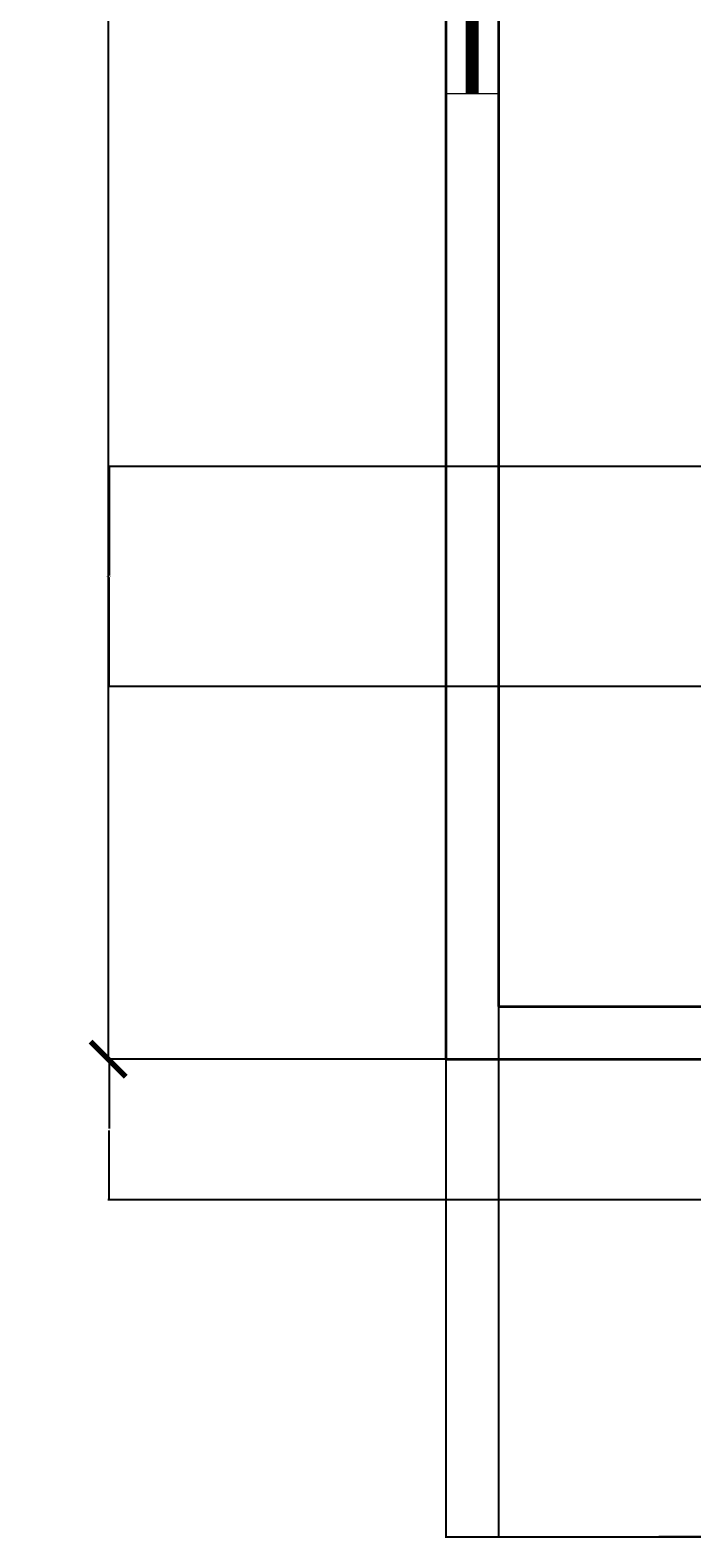
# Model space of a CAD drawing. Units: inches. Extents: x 318 to 927, y -1130 to 13.
# Tile 1 of 17: x 318 to 431, y -1125 to -867. Entities that reach past the tile are written whole.
import ezdxf

# ---------------------------------------------------------------- set-up
doc = ezdxf.new("R2010")
doc.units = ezdxf.units.IN
doc.header["$MEASUREMENT"] = 0
for name, color, linetype, lineweight in [('A-ANNO-DIMS', 1, 'Continuous', 18), ('A-GLAZ-PATT', 5, 'Continuous', 9), ('wall', 1, 'Continuous', 35), ('win', 5, 'Continuous', 18)]:
    doc.layers.add(name, color=color, linetype=linetype, lineweight=lineweight)
doc.styles.get("Standard").update_dxf_attribs({"font": 'arial.ttf'})
doc.dimstyles.get("Standard").update_dxf_attribs({"dimtxt": 0.18, "dimasz": 0.18, "dimexe": 0.18, "dimexo": 0.0625, "dimgap": 0.09, "dimtad": 0, "dimtih": 1, "dimtoh": 1, "dimdec": 1, "dimzin": 0, "dimdsep": 46, "dimlunit": 4, "dimtxsty": 'Standard', "dimcen": 0.09, "dimadec": 0, "dimazin": 0, "dimtfac": 1, "dimtdec": 1, "dimtofl": 0, "dimtmove": 0, "dimatfit": 3, "dimfxl": 1, "dimtolj": 1, "dimtzin": 0, "dimarcsym": 0})

# ---------------------------------------------------------------- blocks, each defined once
blk = doc.blocks.new('_ArchTick')
at = {"color": 0, "linetype": 'ByBlock', "const_width": 0.15}
blk.add_lwpolyline([(-0.5, -0.5), (0.5, 0.5)], dxfattribs=at)
blk = doc.blocks.new('*D4')
at = {"layer": 'A-ANNO-DIMS', "color": 0, "lineweight": -2, "transparency": 16777216}
blk.add_line((331.26, -82.91), (331.26, -1042.91), dxfattribs=at)
at = {"layer": 'Defpoints', "color": 0, "transparency": 16777216}
for p in [(388.89, -82.91), (331.26, -1042.91), (388.89, -1042.91)]:
    blk.add_point(p, dxfattribs=at)
at = {"layer": 'A-ANNO-DIMS', "color": 0, "lineweight": -2, "transparency": 16777216, "xscale": 6, "yscale": 6, "zscale": 6}
for p, rotation in [((331.26, -82.91), 90), ((331.26, -1042.91), 270)]:
    blk.add_blockref('_ArchTick', p, dxfattribs=dict(at, rotation=rotation))
at = {"layer": 'A-ANNO-DIMS', "color": 0, "transparency": 16777216, "insert": (323.18, -562.91), "char_height": 8, "attachment_point": 5, "rotation": 90}
blk.add_mtext("\\A1;80'", dxfattribs=at)
blk = doc.blocks.new('WIN-36IN')
for p, q in [((0, 36), (9, 36)), ((3.5, 36), (3.5, 0)), ((5.5, 36), (5.5, 0)), ((0, 0), (9, 0))]:
    blk.add_line(p, q)
blk = doc.blocks.new('*D26')
at = {"layer": 'A-ANNO-DIMS', "color": 0, "lineweight": -2, "transparency": 16777216}
for p, q in [((645.89, -1042.91), (331.21, -1042.91)), ((331.39, -1043.09), (331.39, -1054.73)), ((331.39, -1066.73), (331.39, -1055.09)), ((645.89, -1066.91), (331.21, -1066.91))]:
    blk.add_line(p, q, dxfattribs=at)
at = {"layer": 'A-ANNO-DIMS', "color": 0, "transparency": 16777216}
for points in [[(331.36, -1043.09), (331.42, -1043.09), (331.39, -1042.91)], [(331.36, -1066.73), (331.42, -1066.73), (331.39, -1066.91)]]:
    blk.add_solid(points, dxfattribs=at)
at = {"layer": 'Defpoints', "color": 0, "transparency": 16777216}
for p in [(645.95, -1042.91), (331.39, -1066.91), (645.95, -1066.91)]:
    blk.add_point(p, dxfattribs=at)
at = {"layer": 'A-ANNO-DIMS', "color": 0, "transparency": 16777216, "insert": (331.39, -1054.91), "char_height": 0.18, "attachment_point": 5}
blk.add_mtext('\\A1;2\'-0"', dxfattribs=at)
blk = doc.blocks.new('*D35')
at = {"layer": 'A-ANNO-DIMS', "color": 0, "lineweight": -2, "transparency": 16777216}
for p, q in [((397.89, -457.98), (397.89, -1124.59)), ((451.89, -457.98), (451.89, -1124.59)), ((398.07, -1124.41), (424.56, -1124.41)), ((451.71, -1124.41), (425.23, -1124.41))]:
    blk.add_line(p, q, dxfattribs=at)
at = {"layer": 'A-ANNO-DIMS', "color": 0, "transparency": 16777216}
for points in [[(398.07, -1124.38), (398.07, -1124.44), (397.89, -1124.41)], [(451.71, -1124.38), (451.71, -1124.44), (451.89, -1124.41)]]:
    blk.add_solid(points, dxfattribs=at)
at = {"layer": 'Defpoints', "color": 0, "transparency": 16777216}
for p in [(397.89, -457.91), (451.89, -457.91), (451.89, -1124.41)]:
    blk.add_point(p, dxfattribs=at)
at = {"layer": 'A-ANNO-DIMS', "color": 0, "transparency": 16777216, "insert": (424.89, -1124.41), "char_height": 0.18, "attachment_point": 5}
blk.add_mtext('\\A1;4\'-6"', dxfattribs=at)
blk = doc.blocks.new('*D55')
at = {"layer": 'A-ANNO-DIMS', "color": 0, "lineweight": -2, "transparency": 16777216}
for p, q in [((833.82, -941.75), (331.21, -941.75)), ((331.39, -941.93), (331.39, -960.35)), ((331.39, -979.13), (331.39, -960.71)), ((833.82, -979.31), (331.21, -979.31))]:
    blk.add_line(p, q, dxfattribs=at)
at = {"layer": 'A-ANNO-DIMS', "color": 0, "transparency": 16777216}
for points in [[(331.36, -941.93), (331.42, -941.93), (331.39, -941.75)], [(331.36, -979.13), (331.42, -979.13), (331.39, -979.31)]]:
    blk.add_solid(points, dxfattribs=at)
at = {"layer": 'Defpoints', "color": 0, "transparency": 16777216}
for p in [(833.89, -941.75), (331.39, -979.31), (833.89, -979.31)]:
    blk.add_point(p, dxfattribs=at)
at = {"layer": 'A-ANNO-DIMS', "color": 0, "transparency": 16777216, "insert": (331.39, -960.53), "char_height": 0.18, "attachment_point": 5}
blk.add_mtext('\\A1;3\'-1 1/2"', dxfattribs=at)
blk = doc.blocks.new('*D71')
at = {"layer": 'A-ANNO-DIMS', "color": 0, "lineweight": -2, "transparency": 16777216}
for p, q in [((388.89, -1042.98), (388.89, -1124.59)), ((547.67, -1042.98), (547.67, -1124.59)), ((389.07, -1124.41), (467.89, -1124.41)), ((547.49, -1124.41), (468.67, -1124.41))]:
    blk.add_line(p, q, dxfattribs=at)
at = {"layer": 'A-ANNO-DIMS', "color": 0, "transparency": 16777216}
for points in [[(389.07, -1124.38), (389.07, -1124.44), (388.89, -1124.41)], [(547.49, -1124.38), (547.49, -1124.44), (547.67, -1124.41)]]:
    blk.add_solid(points, dxfattribs=at)
at = {"layer": 'Defpoints', "color": 0, "transparency": 16777216}
for p in [(388.89, -1042.91), (547.67, -1042.91), (547.67, -1124.41)]:
    blk.add_point(p, dxfattribs=at)
at = {"layer": 'A-ANNO-DIMS', "color": 0, "transparency": 16777216, "insert": (468.28, -1124.41), "char_height": 0.18, "attachment_point": 5}
blk.add_mtext('\\A1;13\'-3"', dxfattribs=at)

msp = doc.modelspace()

# ---------------------------------------------------------------- hatches: boundary and pattern name
at = {"layer": 'A-GLAZ-PATT'}
h = msp.add_hatch(dxfattribs=at)
h.set_pattern_fill('ANSI31', color=256)
h.paths.add_polyline_path([(787.43, -1037.41), (751.43, -1037.41), (751.43, -1039.41), (787.43, -1039.41)])
h.paths.add_polyline_path([(583.67, -1037.41), (547.67, -1037.41), (547.67, -1039.41), (583.67, -1039.41)])
h.paths.add_polyline_path([(394.39, -842.15), (392.39, -842.15), (392.39, -878.15), (394.39, -878.15)])
h.paths.add_polyline_path([(394.39, -788.96), (392.39, -788.96), (392.39, -812.96), (394.39, -812.96)])

# ---------------------------------------------------------------- linework, layer by layer
at = {"layer": 'wall'}
for p, q in [((388.89, -82.91), (388.89, -1042.91)), ((397.89, -829.91), (397.89, -1033.91)), ((397.89, -1033.91), (589.89, -1033.91)), ((388.89, -1042.91), (650.89, -1042.91))]:
    msp.add_line(p, q, dxfattribs=at)

# ---------------------------------------------------------------- block references
at = {"layer": 'win', "rotation": 180}
msp.add_blockref('WIN-36IN', (397.89, -842.15), dxfattribs=at)

# ---------------------------------------------------------------- dimensions: what is measured, and where the dimension line sits
at = {"layer": 'A-ANNO-DIMS'}
for base, p1, p2, override, picture, middle in [((331.26, -1042.91), (388.89, -82.91), (388.89, -1042.91), {"dimtxt": 8, "dimasz": 6, "dimgap": 4, "dimtad": 1, "dimtih": 0, "dimblk1": 'ArchTick', "dimblk2": 'ArchTick', "dimsah": 1, "dimse1": 1, "dimse2": 1, "dimclrd": 0, "dimclre": 0, "dimclrt": 0}, '*D4', (323.18, -562.91)), ((331.39, -979.31), (833.89, -941.75), (833.89, -979.31), {"dimdec": 1, "dimlfac": 1, "dimrnd": 0, "dimzin": 1, "dimdsep": 46, "dimlunit": 4, "dimfrac": 2}, '*D55', (331.39, -960.53)), ((331.39, -1066.91), (645.95, -1042.91), (645.95, -1066.91), {"dimdec": 1, "dimlfac": 1, "dimrnd": 0, "dimzin": 1, "dimdsep": 46, "dimlunit": 4, "dimfrac": 2}, '*D26', (331.39, -1054.91))]:
    dim = msp.add_linear_dim(base=base, p1=p1, p2=p2, angle=90, dimstyle='Standard', override=override, dxfattribs=at)
    dim.commit()
    dim.dimension.update_dxf_attribs({"geometry": picture, "text_midpoint": middle})
for base, p1, p2, picture, middle in [((451.89, -1124.41), (397.89, -457.91), (451.89, -457.91), '*D35', (424.89, -1124.41)), ((547.67, -1124.41), (388.89, -1042.91), (547.67, -1042.91), '*D71', (468.28, -1124.41))]:
    dim = msp.add_linear_dim(base=base, p1=p1, p2=p2, dimstyle='Standard', override={"dimdec": 1, "dimlfac": 1, "dimrnd": 0, "dimzin": 1, "dimdsep": 46, "dimlunit": 4, "dimfrac": 2}, dxfattribs=at)
    dim.commit()
    dim.dimension.update_dxf_attribs({"geometry": picture, "text_midpoint": middle})

doc.saveas('drawing.dxf')
